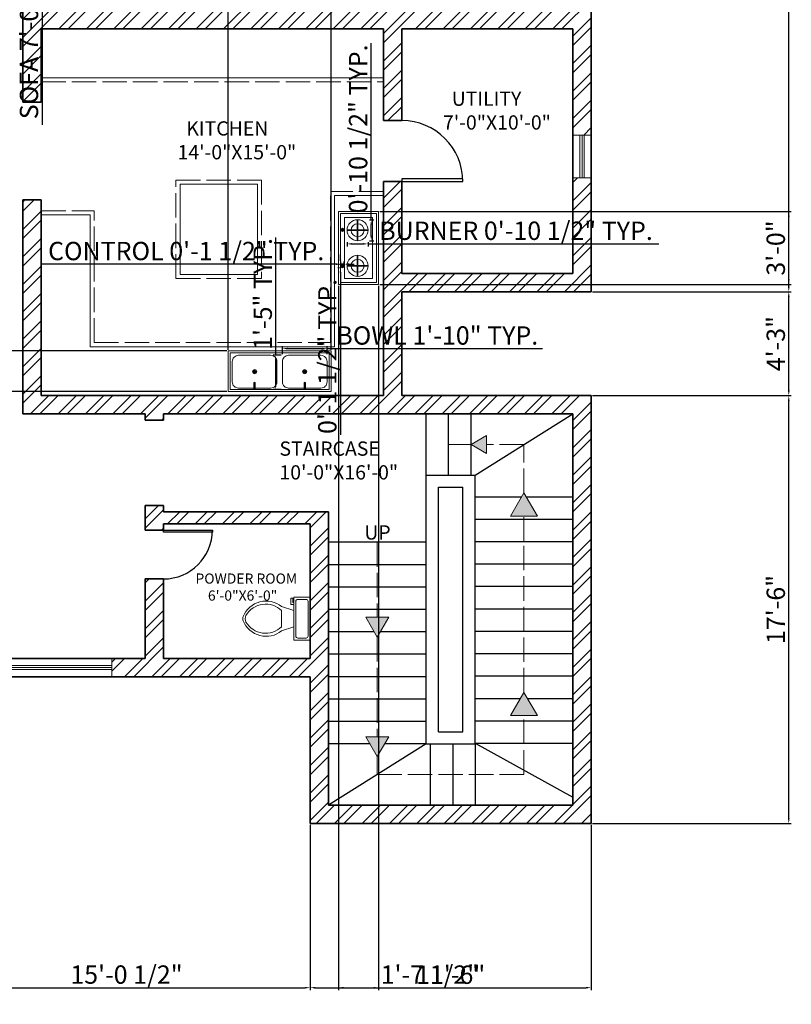
# Model space of a CAD drawing. Units: inches. Extents: x 416 to 1422, y 799 to 1634.
# Tile 4 of 5: x 1043 to 1422, y 799 to 1283. Entities that reach past the tile are written whole.
import ezdxf

# ---------------------------------------------------------------- set-up
doc = ezdxf.new("R2010")
doc.units = ezdxf.units.IN
doc.linetypes.add('ACAD_ISO02W100', pattern=[15, 12, -3])
for name, color, linetype, lineweight in [('A-ANNO-DIMS', 2, 'Continuous', 18), ('A-ANNO-STRS-PATH', 7, 'ACAD_ISO02W100', 18), ('A-ANNO-SYMB', 7, 'Continuous', 18), ('A-ANNO-TEXT', 7, 'Continuous', 18), ('A-AREA-IDEN', 7, 'Continuous', 18), ('A-DOOR', 4, 'Continuous', 25), ('A-EQPM', 9, 'Continuous', 18), ('A-FLOR-CASE', 8, 'Continuous', 18), ('A-FLOR-CASE-HIDN', 8, 'ACAD_ISO02W100', 13), ('A-FLOR-FIXT', 9, 'Continuous', 18), ('A-FLOR-STRS', 7, 'Continuous', 25), ('A-GLAZ', 244, 'Continuous', 18), ('A-WALL', 7, 'Continuous', 35), ('A-WALL-PATT', 252, 'Continuous', 13)]:
    doc.layers.add(name, color=color, linetype=linetype, lineweight=lineweight)
doc.styles.get("Standard").update_dxf_attribs({"font": 'arial.ttf'})
doc.dimstyles.new('ISO-25', dxfattribs={"dimtxt": 9, "dimasz": 2.5, "dimexe": 1.25, "dimexo": 0.625, "dimtad": 1, "dimlunit": 3, "dimtxsty": 'Standard', "dimcen": 2.5, "dimadec": 0, "dimazin": 0, "dimtfac": 1, "dimtmove": 0, "dimatfit": 3, "dimfxl": 1, "dimarcsym": 0})

# ---------------------------------------------------------------- blocks, each defined once
blk = doc.blocks.new('*U3')
for p, q in [((-40, 0), (-40, 6)), ((0, 0), (0, 6))]:
    blk.add_line(p, q)
blk.add_lwpolyline([(0, 0), (0, -40), (-1.75, -40), (-1.75, 0)], close=True)
blk.add_arc((0, 0), 40, 180, 270)
blk = doc.blocks.new('*U7')
for p, q in [((9.5, -6), (9.5, -2)), ((-10, -8.5), (-8, -8.5)), ((-10, -9.5), (-10, -8.5)), ((-7, -9.5), (-10, -9.5)), ((-8, -8.5), (-8, -8)), ((-7, -8), (-7, -9.5)), ((-4, -8), (-6, -14)), ((4, -8), (6, -14)), ((4, -14), (-4, -14))]:
    blk.add_line(p, q)
blk.add_lwpolyline([(10.5, -8), (10.5, 0), (-10.5, 0), (-10.5, -8)], close=True)
for points in [[(-9.5, -2), (-9.5, -6)], [(8.5, -1), (-8.5, -1)], [(-8.5, -7), (8.5, -7)]]:
    blk.add_lwpolyline(points)
for centre, radius, start, end in [((-8.62, -1.88), 0.884, 81.8699, 188.1301), ((8.62, -1.88), 0.884, 351.8699, 98.1301), ((-8.62, -6.12), 0.884, 171.8699, 278.1301), ((8.62, -6.12), 0.884, 261.8699, 8.1301), ((3.52, -21.58), 12.17, 141.4691, 247.9714), ((4.2, -21.82), 11.33, 136.3677, 238.9468), ((-3.52, -21.58), 12.17, 292.0284, 38.5307), ((-4.2, -21.82), 11.33, 301.053, 43.6321), ((0, -27.88), 4, 245.7318, 294.2682), ((0, -29), 4, 254.8605, 285.1395)]:
    blk.add_arc(centre, radius, start, end)
blk = doc.blocks.new('*U9')
for p, q in [((0, 0), (0, 6)), ((40, 0), (40, 6))]:
    blk.add_line(p, q)
blk.add_lwpolyline([(0, 0), (0, -40), (1.75, -40), (1.75, 0)], close=True)
blk.add_arc((0, 0), 40, 270, 360)
blk = doc.blocks.new('WIN-21IN')
for p, q in [((21, 5.5), (0, 5.5)), ((21, 4.5), (0, 4.5)), ((21, 3.5), (0, 3.5))]:
    blk.add_line(p, q)
blk.add_lwpolyline([(21, 9), (21, 0), (0, 0), (0, 9)], close=True)
blk = doc.blocks.new('WIN-60IN')
for p, q in [((3.5, 60), (3.5, 0)), ((4.5, 60), (4.5, 0)), ((5.5, 60), (5.5, 0))]:
    blk.add_line(p, q)
blk.add_lwpolyline([(0, 60), (9, 60), (9, 0), (0, 0)], close=True)
blk = doc.blocks.new('SINK-BOWL-WITH-DRAIN')
for p, q in [((10.95, 9.8), (10.95, 7.77)), ((9.94, 8.78), (11.97, 8.78)), ((10.22, 9.49), (11.68, 8.08)), ((11.67, 9.5), (10.23, 8.07)), ((10.71, 0), (10.71, 2.96)), ((10.81, 0), (10.81, 2.87)), ((11.21, 0), (11.21, 2.86)), ((11.31, 0), (11.31, 2.94))]:
    blk.add_line(p, q)
blk.add_lwpolyline([(10.71, 0.74), (3, 0.74, -0.414214), (0, 3.74), (0, 13.82, -0.414214), (3, 16.82), (18.91, 16.82, -0.414214), (21.91, 13.82), (21.91, 3.74, -0.414214), (18.91, 0.74), (11.31, 0.74)], format="xyb")
for centre, radius in [((10.95, 8.78), 1.02), ((10.95, 8.78), 0.616), ((11.02, 3.19), 0.381), ((11.02, 3.19), 0.181)]:
    blk.add_circle(centre, radius)
blk = doc.blocks.new('COOKTOP-BURNER')
for p, q in [((4.97, 10.34), (4.97, 5.37)), ((5.37, 10.34), (5.37, 5.37)), ((4.97, 5.37), (0, 5.37)), ((4.97, 4.97), (0, 4.97)), ((3.97, 5.37), (3.97, 4.97)), ((5.37, 6.37), (4.97, 6.37)), ((4.97, 4.97), (4.97, 0)), ((10.34, 5.37), (5.37, 5.37)), ((10.34, 4.97), (5.37, 4.97)), ((5.37, 4.97), (5.37, 0)), ((6.37, 5.37), (6.37, 4.97)), ((5.37, 3.97), (4.97, 3.97))]:
    blk.add_line(p, q)
for radius in [5.17, 3.17]:
    blk.add_circle((5.17, 5.17), radius)
blk = doc.blocks.new('COOKTOP-CONTROL')
for p, q in [((0.56, 1.39), (0.56, 0.13)), ((0.96, 1.39), (0.96, 0.13))]:
    blk.add_line(p, q)
for radius in [0.761, 0.661]:
    blk.add_circle((0.76, 0.76), radius)
blk = doc.blocks.new('*D27')
at = {"layer": 'A-ANNO-DIMS', "color": 0, "lineweight": -2, "transparency": 16777216}
for p, q in [((1042.27, 1411.23), (1055.49, 1411.23)), ((1054.24, 1408.73), (1054.24, 1329.73)), ((1042.27, 1327.23), (1055.49, 1327.23)), ((1054.24, 1327.23), (1054.24, 1230.94))]:
    blk.add_line(p, q, dxfattribs=at)
at = {"layer": 'A-ANNO-DIMS', "color": 0, "transparency": 16777216}
for points in [[(1053.83, 1408.73), (1054.66, 1408.73), (1054.24, 1411.23)], [(1053.83, 1329.73), (1054.66, 1329.73), (1054.24, 1327.23)]]:
    blk.add_solid(points, dxfattribs=at)
at = {"layer": 'Defpoints', "color": 0, "transparency": 16777216}
for p in [(1041.64, 1411.23), (1041.64, 1327.23), (1054.24, 1327.23)]:
    blk.add_point(p, dxfattribs=at)
at = {"layer": 'A-ANNO-DIMS', "color": 0, "transparency": 16777216, "insert": (1048.96, 1277.83), "char_height": 9, "attachment_point": 5, "rotation": 90}
blk.add_mtext('SOFA 7\'-0" TYP.', dxfattribs=at)
blk = doc.blocks.new('*D35')
at = {"layer": 'A-ANNO-DIMS', "color": 0, "lineweight": -2, "transparency": 16777216}
for p, q in [((1172.23, 1118.41), (1172.23, 1122.32)), ((1194.14, 1118.41), (1194.14, 1122.32)), ((1174.73, 1121.07), (1191.64, 1121.07)), ((1194.14, 1121.07), (1299.86, 1121.07))]:
    blk.add_line(p, q, dxfattribs=at)
at = {"layer": 'A-ANNO-DIMS', "color": 0, "transparency": 16777216}
for points in [[(1174.73, 1121.48), (1174.73, 1120.65), (1172.23, 1121.07)], [(1191.64, 1121.48), (1191.64, 1120.65), (1194.14, 1121.07)]]:
    blk.add_solid(points, dxfattribs=at)
at = {"layer": 'Defpoints', "color": 0, "transparency": 16777216}
for p in [(1172.23, 1117.78), (1194.14, 1121.07), (1194.14, 1117.78)]:
    blk.add_point(p, dxfattribs=at)
at = {"layer": 'A-ANNO-DIMS', "color": 0, "transparency": 16777216, "insert": (1248.25, 1126.35), "char_height": 9, "attachment_point": 5}
blk.add_mtext('BOWL 1\'-10" TYP.', dxfattribs=at)
blk = doc.blocks.new('*D36')
at = {"layer": 'A-ANNO-DIMS', "color": 0, "lineweight": -2, "transparency": 16777216}
for p, q in [((1168.94, 1117.78), (1168.94, 1175.54)), ((1171.6, 1117.78), (1167.69, 1117.78)), ((1168.94, 1103.46), (1168.94, 1115.28)), ((1171.6, 1100.96), (1167.69, 1100.96))]:
    blk.add_line(p, q, dxfattribs=at)
at = {"layer": 'A-ANNO-DIMS', "color": 0, "transparency": 16777216}
for points in [[(1168.53, 1115.28), (1169.36, 1115.28), (1168.94, 1117.78)], [(1168.53, 1103.46), (1169.36, 1103.46), (1168.94, 1100.96)]]:
    blk.add_solid(points, dxfattribs=at)
at = {"layer": 'Defpoints', "color": 0, "transparency": 16777216}
for p in [(1168.94, 1117.78), (1172.23, 1117.78), (1172.23, 1100.96)]:
    blk.add_point(p, dxfattribs=at)
at = {"layer": 'A-ANNO-DIMS', "color": 0, "transparency": 16777216, "insert": (1163.72, 1147.91), "char_height": 9, "attachment_point": 5, "rotation": 90}
blk.add_mtext('1\'-5" TYP.', dxfattribs=at)
blk = doc.blocks.new('*D37')
at = {"layer": 'A-ANNO-DIMS', "color": 0, "lineweight": -2, "transparency": 16777216}
for p, q in [((1203.95, 1173.39), (1203.95, 1171.22)), ((1206.45, 1172.47), (1211.78, 1172.47)), ((1214.28, 1173.39), (1214.28, 1171.22)), ((1214.28, 1172.47), (1357.04, 1172.47))]:
    blk.add_line(p, q, dxfattribs=at)
at = {"layer": 'A-ANNO-DIMS', "color": 0, "transparency": 16777216}
for points in [[(1206.45, 1172.88), (1206.45, 1172.05), (1203.95, 1172.47)], [(1211.78, 1172.88), (1211.78, 1172.05), (1214.28, 1172.47)]]:
    blk.add_solid(points, dxfattribs=at)
at = {"layer": 'Defpoints', "color": 0, "transparency": 16777216}
for p in [(1203.95, 1174.02), (1214.28, 1174.02), (1214.28, 1172.47)]:
    blk.add_point(p, dxfattribs=at)
at = {"layer": 'A-ANNO-DIMS', "color": 0, "transparency": 16777216, "insert": (1286.91, 1177.75), "char_height": 9, "attachment_point": 5}
blk.add_mtext('BURNER 0\'-10 1/2" TYP.', dxfattribs=at)
blk = doc.blocks.new('*D38')
at = {"layer": 'A-ANNO-DIMS', "color": 0, "lineweight": -2, "transparency": 16777216}
for p, q in [((1215.83, 1184.35), (1215.83, 1270.93)), ((1214.91, 1184.35), (1217.08, 1184.35)), ((1215.83, 1176.52), (1215.83, 1181.85)), ((1214.91, 1174.02), (1217.08, 1174.02))]:
    blk.add_line(p, q, dxfattribs=at)
at = {"layer": 'A-ANNO-DIMS', "color": 0, "transparency": 16777216}
for points in [[(1215.42, 1181.85), (1216.25, 1181.85), (1215.83, 1184.35)], [(1215.42, 1176.52), (1216.25, 1176.52), (1215.83, 1174.02)]]:
    blk.add_solid(points, dxfattribs=at)
at = {"layer": 'Defpoints', "color": 0, "transparency": 16777216}
for p in [(1214.28, 1184.35), (1215.83, 1184.35), (1214.28, 1174.02)]:
    blk.add_point(p, dxfattribs=at)
at = {"layer": 'A-ANNO-DIMS', "color": 0, "transparency": 16777216, "insert": (1210.56, 1228.89), "char_height": 9, "attachment_point": 5, "rotation": 90}
blk.add_mtext('0\'-10 1/2" TYP.', dxfattribs=at)
blk = doc.blocks.new('*D39')
at = {"layer": 'A-ANNO-DIMS', "color": 0, "lineweight": -2, "transparency": 16777216}
for p, q in [((1198.45, 1162.52), (1054, 1162.52)), ((1200.95, 1162.91), (1200.95, 1163.77)), ((1202.47, 1162.52), (1200.95, 1162.52)), ((1202.47, 1162.91), (1202.47, 1163.77)), ((1204.97, 1162.52), (1207.47, 1162.52))]:
    blk.add_line(p, q, dxfattribs=at)
at = {"layer": 'A-ANNO-DIMS', "color": 0, "transparency": 16777216}
for points in [[(1198.45, 1162.93), (1198.45, 1162.1), (1200.95, 1162.52)], [(1204.97, 1162.93), (1204.97, 1162.1), (1202.47, 1162.52)]]:
    blk.add_solid(points, dxfattribs=at)
at = {"layer": 'Defpoints', "color": 0, "transparency": 16777216}
for p in [(1200.95, 1162.52), (1200.95, 1162.29), (1202.47, 1162.29)]:
    blk.add_point(p, dxfattribs=at)
at = {"layer": 'A-ANNO-DIMS', "color": 0, "transparency": 16777216, "insert": (1124.98, 1167.8), "char_height": 9, "attachment_point": 5}
blk.add_mtext('CONTROL 0\'-1 1/2" TYP.', dxfattribs=at)
blk = doc.blocks.new('*D40')
at = {"layer": 'A-ANNO-DIMS', "color": 0, "lineweight": -2, "transparency": 16777216}
for p, q in [((1200.72, 1164.79), (1200.72, 1167.29)), ((1200.32, 1162.29), (1199.47, 1162.29)), ((1200.32, 1160.77), (1199.47, 1160.77)), ((1200.72, 1162.29), (1200.72, 1160.77)), ((1200.72, 1158.27), (1200.72, 1078.69))]:
    blk.add_line(p, q, dxfattribs=at)
at = {"layer": 'A-ANNO-DIMS', "color": 0, "transparency": 16777216}
for points in [[(1200.3, 1164.79), (1201.13, 1164.79), (1200.72, 1162.29)], [(1200.3, 1158.27), (1201.13, 1158.27), (1200.72, 1160.77)]]:
    blk.add_solid(points, dxfattribs=at)
at = {"layer": 'Defpoints', "color": 0, "transparency": 16777216}
for p in [(1200.72, 1160.77), (1200.95, 1162.29), (1200.95, 1160.77)]:
    blk.add_point(p, dxfattribs=at)
at = {"layer": 'A-ANNO-DIMS', "color": 0, "transparency": 16777216, "insert": (1195.44, 1117.23), "char_height": 9, "attachment_point": 5, "rotation": 90}
blk.add_mtext('0\'-1 1/2" TYP.', dxfattribs=at)
blk = doc.blocks.new('*D46')
at = {"layer": 'A-ANNO-DIMS', "color": 0, "lineweight": -2, "transparency": 16777216}
for p, q in [((1185.82, 887.39), (1185.82, 806.13)), ((1005.49, 855.39), (1005.49, 806.13)), ((1007.99, 807.38), (1183.32, 807.38))]:
    blk.add_line(p, q, dxfattribs=at)
at = {"layer": 'A-ANNO-DIMS', "color": 0, "transparency": 16777216}
for points in [[(1007.99, 807.79), (1007.99, 806.96), (1005.49, 807.38)], [(1183.32, 807.79), (1183.32, 806.96), (1185.82, 807.38)]]:
    blk.add_solid(points, dxfattribs=at)
at = {"layer": 'Defpoints', "color": 0, "transparency": 16777216}
for p in [(1185.82, 888.01), (1005.49, 856.01), (1185.82, 807.38)]:
    blk.add_point(p, dxfattribs=at)
at = {"layer": 'A-ANNO-DIMS', "color": 0, "transparency": 16777216, "insert": (1095.65, 812.65), "char_height": 9, "attachment_point": 5}
blk.add_mtext('15\'-0 1/2"', dxfattribs=at)
blk = doc.blocks.new('*D47')
at = {"layer": 'A-ANNO-DIMS', "color": 0, "lineweight": -2, "transparency": 16777216}
for p, q in [((1185.82, 887.39), (1185.82, 806.13)), ((1323.82, 887.39), (1323.82, 806.13)), ((1188.32, 807.38), (1321.32, 807.38))]:
    blk.add_line(p, q, dxfattribs=at)
at = {"layer": 'A-ANNO-DIMS', "color": 0, "transparency": 16777216}
for points in [[(1188.32, 807.79), (1188.32, 806.96), (1185.82, 807.38)], [(1321.32, 807.79), (1321.32, 806.96), (1323.82, 807.38)]]:
    blk.add_solid(points, dxfattribs=at)
at = {"layer": 'Defpoints', "color": 0, "transparency": 16777216}
for p in [(1185.82, 888.01), (1323.82, 888.01), (1323.82, 807.38)]:
    blk.add_point(p, dxfattribs=at)
at = {"layer": 'A-ANNO-DIMS', "color": 0, "transparency": 16777216, "insert": (1254.82, 812.6), "char_height": 9, "attachment_point": 5}
blk.add_mtext('11\'-6"', dxfattribs=at)
blk = doc.blocks.new('*D48')
at = {"layer": 'A-ANNO-DIMS', "color": 0, "lineweight": -2, "transparency": 16777216}
for p, q in [((1324.44, 1098.01), (1422.07, 1098.01)), ((1420.82, 890.51), (1420.82, 1095.51)), ((1324.44, 888.01), (1422.07, 888.01))]:
    blk.add_line(p, q, dxfattribs=at)
at = {"layer": 'A-ANNO-DIMS', "color": 0, "transparency": 16777216}
for points in [[(1420.4, 1095.51), (1421.24, 1095.51), (1420.82, 1098.01)], [(1420.4, 890.51), (1421.24, 890.51), (1420.82, 888.01)]]:
    blk.add_solid(points, dxfattribs=at)
at = {"layer": 'Defpoints', "color": 0, "transparency": 16777216}
for p in [(1323.82, 1098.01), (1420.82, 1098.01), (1323.82, 888.01)]:
    blk.add_point(p, dxfattribs=at)
at = {"layer": 'A-ANNO-DIMS', "color": 0, "transparency": 16777216, "insert": (1415.6, 993.01), "char_height": 9, "attachment_point": 5, "rotation": 90}
blk.add_mtext('17\'-6"', dxfattribs=at)
blk = doc.blocks.new('*D49')
at = {"layer": 'A-ANNO-DIMS', "color": 0, "lineweight": -2, "transparency": 16777216}
for p, q in [((1324.44, 1149.01), (1422.07, 1149.01)), ((1420.82, 1100.51), (1420.82, 1146.51)), ((1324.44, 1098.01), (1422.07, 1098.01))]:
    blk.add_line(p, q, dxfattribs=at)
at = {"layer": 'A-ANNO-DIMS', "color": 0, "transparency": 16777216}
for points in [[(1420.4, 1146.51), (1421.24, 1146.51), (1420.82, 1149.01)], [(1420.4, 1100.51), (1421.24, 1100.51), (1420.82, 1098.01)]]:
    blk.add_solid(points, dxfattribs=at)
at = {"layer": 'Defpoints', "color": 0, "transparency": 16777216}
for p in [(1323.82, 1149.01), (1420.82, 1149.01), (1323.82, 1098.01)]:
    blk.add_point(p, dxfattribs=at)
at = {"layer": 'A-ANNO-DIMS', "color": 0, "transparency": 16777216, "insert": (1415.6, 1123.51), "char_height": 9, "attachment_point": 5, "rotation": 90}
blk.add_mtext('4\'-3"', dxfattribs=at)
blk = doc.blocks.new('*D50')
at = {"layer": 'A-ANNO-DIMS', "color": 0, "lineweight": -2, "transparency": 16777216}
for p, q in [((1324.44, 1569.01), (1422.07, 1569.01)), ((1420.82, 1151.51), (1420.82, 1566.51)), ((1324.44, 1149.01), (1422.07, 1149.01))]:
    blk.add_line(p, q, dxfattribs=at)
at = {"layer": 'A-ANNO-DIMS', "color": 0, "transparency": 16777216}
for points in [[(1420.4, 1566.51), (1421.24, 1566.51), (1420.82, 1569.01)], [(1420.4, 1151.51), (1421.24, 1151.51), (1420.82, 1149.01)]]:
    blk.add_solid(points, dxfattribs=at)
at = {"layer": 'Defpoints', "color": 0, "transparency": 16777216}
for p in [(1323.82, 1569.01), (1420.82, 1569.01), (1323.82, 1149.01)]:
    blk.add_point(p, dxfattribs=at)
at = {"layer": 'A-ANNO-DIMS', "color": 0, "transparency": 16777216, "insert": (1415.6, 1359.01), "char_height": 9, "attachment_point": 5, "rotation": 90}
blk.add_mtext('35\'-0"', dxfattribs=at)
blk = doc.blocks.new('*D54')
at = {"layer": 'A-ANNO-DIMS', "color": 0, "lineweight": -2, "transparency": 16777216}
for p, q in [((1199.73, 1151.87), (1199.73, 806.13)), ((1219.46, 1151.87), (1219.46, 806.13)), ((1202.23, 807.38), (1216.96, 807.38)), ((1219.46, 807.38), (1267.26, 807.38))]:
    blk.add_line(p, q, dxfattribs=at)
at = {"layer": 'A-ANNO-DIMS', "color": 0, "transparency": 16777216}
for points in [[(1202.23, 807.79), (1202.23, 806.96), (1199.73, 807.38)], [(1216.96, 807.79), (1216.96, 806.96), (1219.46, 807.38)]]:
    blk.add_solid(points, dxfattribs=at)
at = {"layer": 'Defpoints', "color": 0, "transparency": 16777216}
for p in [(1199.73, 1152.5), (1219.46, 1152.5), (1219.46, 807.38)]:
    blk.add_point(p, dxfattribs=at)
at = {"layer": 'A-ANNO-DIMS', "color": 0, "transparency": 16777216, "insert": (1244.61, 812.65), "char_height": 9, "attachment_point": 5}
blk.add_mtext('1\'-7 1/2"', dxfattribs=at)
blk = doc.blocks.new('*D55')
at = {"layer": 'A-ANNO-DIMS', "color": 0, "lineweight": -2, "transparency": 16777216}
for p, q in [((1220.08, 1188.39), (1422.07, 1188.39)), ((1420.82, 1155), (1420.82, 1185.89)), ((1220.08, 1152.5), (1422.07, 1152.5))]:
    blk.add_line(p, q, dxfattribs=at)
at = {"layer": 'A-ANNO-DIMS', "color": 0, "transparency": 16777216}
for points in [[(1420.4, 1185.89), (1421.24, 1185.89), (1420.82, 1188.39)], [(1420.4, 1155), (1421.24, 1155), (1420.82, 1152.5)]]:
    blk.add_solid(points, dxfattribs=at)
at = {"layer": 'Defpoints', "color": 0, "transparency": 16777216}
for p in [(1219.46, 1188.39), (1420.82, 1188.39), (1219.46, 1152.5)]:
    blk.add_point(p, dxfattribs=at)
at = {"layer": 'A-ANNO-DIMS', "color": 0, "transparency": 16777216, "insert": (1415.6, 1170.44), "char_height": 9, "attachment_point": 5, "rotation": 90}
blk.add_mtext('3\'-0"', dxfattribs=at)
blk = doc.blocks.new('*D56')
at = {"layer": 'A-ANNO-DIMS', "color": 0, "lineweight": -2, "transparency": 16777216}
for p, q in [((1145.53, 1120.54), (1145.53, 1616.26)), ((1148.03, 1615.01), (1193.73, 1615.01)), ((1196.23, 1120.54), (1196.23, 1616.26))]:
    blk.add_line(p, q, dxfattribs=at)
at = {"layer": 'A-ANNO-DIMS', "color": 0, "transparency": 16777216}
for points in [[(1148.03, 1615.43), (1148.03, 1614.6), (1145.53, 1615.01)], [(1193.73, 1615.43), (1193.73, 1614.6), (1196.23, 1615.01)]]:
    blk.add_solid(points, dxfattribs=at)
at = {"layer": 'Defpoints', "color": 0, "transparency": 16777216}
for p in [(1196.23, 1615.01), (1145.53, 1119.92), (1196.23, 1119.92)]:
    blk.add_point(p, dxfattribs=at)
at = {"layer": 'A-ANNO-DIMS', "color": 0, "transparency": 16777216, "insert": (1170.88, 1620.29), "char_height": 9, "attachment_point": 5}
blk.add_mtext('4\'-2 1/2"', dxfattribs=at)
blk = doc.blocks.new('*D57')
at = {"layer": 'A-ANNO-DIMS', "color": 0, "lineweight": -2, "transparency": 16777216}
for p, q in [((434.25, 1119.92), (434.25, 1146.74)), ((1144.9, 1119.92), (433, 1119.92)), ((434.25, 1102.46), (434.25, 1117.42)), ((1144.9, 1099.96), (433, 1099.96))]:
    blk.add_line(p, q, dxfattribs=at)
at = {"layer": 'A-ANNO-DIMS', "color": 0, "transparency": 16777216}
for points in [[(433.83, 1117.42), (434.67, 1117.42), (434.25, 1119.92)], [(433.83, 1102.46), (434.67, 1102.46), (434.25, 1099.96)]]:
    blk.add_solid(points, dxfattribs=at)
at = {"layer": 'Defpoints', "color": 0, "transparency": 16777216}
for p in [(434.25, 1119.92), (1145.53, 1119.92), (1145.53, 1099.96)]:
    blk.add_point(p, dxfattribs=at)
at = {"layer": 'A-ANNO-DIMS', "color": 0, "transparency": 16777216, "insert": (429.03, 1134.58), "char_height": 9, "attachment_point": 5, "rotation": 90}
blk.add_mtext('1\'-8"', dxfattribs=at)

msp = doc.modelspace()

# ---------------------------------------------------------------- hatches: boundary and pattern name
at = {"layer": 'A-ANNO-SYMB'}
h = msp.add_hatch(color=256, dxfattribs=at)
h.dxf.hatch_style = 1
h.paths.add_polyline_path([(1224.457, 989.211), (1213.183, 989.211), (1218.82, 979.448)])
h.paths.add_polyline_path([(1224.457, 930.584), (1213.183, 930.584), (1218.82, 920.821)])
h.paths.add_polyline_path([(1290.82, 952.305), (1284.259, 940.942), (1297.38, 940.942)])
h.paths.add_polyline_path([(1290.82, 1050.204), (1284.259, 1038.841), (1297.38, 1038.841)])
h.paths.add_polyline_path([(1272.477, 1078.434), (1264.82, 1074.013), (1272.477, 1069.591)])
at = {"layer": 'A-WALL-PATT'}
h = msp.add_hatch(dxfattribs=at)
h.set_pattern_fill('ANSI32', color=256)
h.paths.add_polyline_path([(695.32, 1569.013), (607.303, 1569.013), (607.303, 1560.013), (660.82, 1560.013), (660.82, 1419.013), (657.82, 1419.013), (657.82, 1413.013), (669.82, 1413.013), (669.82, 1446.013), (672.82, 1446.013), (672.82, 1452.013), (669.82, 1452.013), (669.82, 1560.013), (695.32, 1560.013)])
h.paths.add_polyline_path([(1323.82, 1311.283), (1314.82, 1311.283), (1314.82, 1287.013), (1242.82, 1287.013), (1242.82, 1383.013), (1245.82, 1383.013), (1245.82, 1392.013), (1236.82, 1392.013), (1236.82, 1339.513), (1158.82, 1339.513), (1158.82, 1431.013), (1149.82, 1431.013), (1149.82, 1287.013), (1044.82, 1287.013), (1044.82, 1242.013), (1053.82, 1242.013), (1053.82, 1278.013), (1221.82, 1278.013), (1221.82, 1233.013), (1230.82, 1233.013), (1230.82, 1278.013), (1314.82, 1278.013), (1314.82, 1225.894), (1323.82, 1225.894)])
h.paths.add_polyline_path([(1158.82, 1287.013), (1158.82, 1333.513), (1236.82, 1333.513), (1236.82, 1287.013)], flags=16)
h.paths.add_polyline_path([(1323.82, 1569.013), (1283.747, 1569.013), (1283.747, 1560.013), (1314.82, 1560.013), (1314.82, 1392.013), (1275.82, 1392.013), (1275.82, 1383.013), (1314.82, 1383.013), (1314.82, 1332.283), (1323.82, 1332.283)])
h.paths.add_polyline_path([(750.82, 1569.013), (716.32, 1569.013), (716.32, 1560.013), (741.82, 1560.013), (741.82, 1452.013), (702.82, 1452.013), (702.82, 1447.513), (702.82, 1446.013), (741.82, 1446.013), (741.82, 1287.013), (750.82, 1287.013)])
h.paths.add_polyline_path([(1158.82, 1560.013), (1223.747, 1560.013), (1223.747, 1569.013), (1149.82, 1569.013), (1149.82, 1467.013), (1158.82, 1467.013)])
h.paths.add_polyline_path([(1323.82, 1098.013), (1230.82, 1098.013), (1230.82, 1149.013), (1323.82, 1149.013), (1323.82, 1204.894), (1314.82, 1204.894), (1314.82, 1158.013), (1230.82, 1158.013), (1230.82, 1203.013), (1221.82, 1203.013), (1221.82, 1098.013), (1053.82, 1098.013), (1053.82, 1194.013), (1044.82, 1194.013), (1044.82, 1089.013), (1104.82, 1089.013), (1104.82, 1086.013), (1113.82, 1086.013), (1113.82, 1089.013), (1194.82, 1089.013), (1314.82, 1089.013), (1314.82, 897.013), (1194.82, 897.013), (1194.82, 1041.013), (1113.82, 1041.013), (1113.82, 1044.013), (1104.82, 1044.013), (1104.82, 1032.013), (1113.82, 1032.013), (1113.82, 1035.013), (1185.82, 1035.013), (1185.82, 969.013), (1113.82, 969.013), (1113.82, 1008.013), (1104.82, 1008.013), (1104.82, 969.013), (1088.452, 969.013), (1088.452, 960.013), (1185.82, 960.013), (1185.82, 888.013), (1323.82, 888.013)])

# ---------------------------------------------------------------- linework, layer by layer
at = {"layer": 'A-ANNO-STRS-PATH'}
for p, q in [((1264.82, 1074.013), (1253.82, 1074.013)), ((1290.82, 1074.013), (1272.477, 1074.013)), ((1290.82, 1050.204), (1290.82, 1074.013)), ((1290.82, 1026.395), (1290.82, 1038.841)), ((1218.82, 1026.013), (1218.82, 989.211)), ((1290.82, 952.305), (1290.82, 1026.395)), ((1218.82, 979.448), (1218.82, 930.584)), ((1290.82, 912.013), (1290.82, 940.942)), ((1218.82, 920.821), (1218.82, 912.013)), ((1218.82, 912.013), (1290.82, 912.013))]:
    msp.add_line(p, q, dxfattribs=at)
at = {"layer": 'A-ANNO-SYMB'}
for points in [[(1264.82, 1074.013), (1272.477, 1069.591), (1272.477, 1078.434)], [(1290.82, 1050.204), (1284.259, 1038.841), (1297.38, 1038.841)], [(1218.82, 979.448), (1224.457, 989.211), (1213.183, 989.211)], [(1290.82, 952.305), (1284.259, 940.942), (1297.38, 940.942)], [(1218.82, 920.821), (1224.457, 930.584), (1213.183, 930.584)]]:
    msp.add_lwpolyline(points, close=True, dxfattribs=at)
at = {"layer": 'A-EQPM'}
for points in [[(1199.726, 1188.394), (1219.46, 1188.394), (1219.46, 1152.496), (1199.726, 1152.496)], [(1200.726, 1187.394), (1218.46, 1187.394), (1218.46, 1153.496), (1200.726, 1153.496)], [(1202.726, 1185.394), (1216.46, 1185.394), (1216.46, 1155.496), (1202.726, 1155.496)]]:
    msp.add_lwpolyline(points, close=True, dxfattribs=at)
at = {"layer": 'A-FLOR-CASE'}
for p, q in [((1053.82, 1254.013), (1221.82, 1254.013)), ((1197.82, 1122.013), (1197.82, 1196.185)), ((1221.82, 1196.185), (1197.82, 1196.185)), ((1053.82, 1186.76), (1077.82, 1186.76)), ((1077.82, 1122.013), (1077.82, 1186.76)), ((1077.82, 1122.013), (1197.82, 1122.013))]:
    msp.add_line(p, q, dxfattribs=at)
msp.add_lwpolyline([(1121.959, 1201.774), (1159.95, 1201.774), (1159.95, 1157.434), (1121.959, 1157.434)], close=True, dxfattribs=at)
at = {"layer": 'A-FLOR-CASE-HIDN'}
for p, q in [((1053.82, 1252.013), (1221.82, 1252.013)), ((1221.82, 1198.185), (1195.82, 1198.185)), ((1195.82, 1124.013), (1195.82, 1198.185)), ((1053.82, 1188.76), (1079.82, 1188.76)), ((1079.82, 1124.013), (1079.82, 1188.76)), ((1079.82, 1124.013), (1195.82, 1124.013))]:
    msp.add_line(p, q, dxfattribs=at)
msp.add_lwpolyline([(1119.959, 1203.774), (1161.95, 1203.774), (1161.95, 1155.434), (1119.959, 1155.434)], close=True, dxfattribs=at)
at = {"layer": 'A-FLOR-FIXT'}
for points in [[(1145.527, 1119.918), (1196.227, 1119.918), (1196.227, 1099.958), (1145.527, 1099.958)], [(1146.527, 1118.918), (1195.227, 1118.918), (1195.227, 1100.958), (1146.527, 1100.958)]]:
    msp.add_lwpolyline(points, close=True, dxfattribs=at)
at = {"layer": 'A-FLOR-STRS'}
for p, q in [((1242.82, 1059.013), (1242.82, 1089.013)), ((1253.82, 1059.013), (1253.82, 1089.013)), ((1264.82, 1059.013), (1264.82, 1089.013)), ((1266.82, 1059.013), (1314.82, 1089.013)), ((1242.82, 927.013), (1242.82, 1059.013)), ((1242.82, 1059.013), (1266.82, 1059.013)), ((1266.82, 927.013), (1266.82, 1059.013)), ((1248.82, 933.013), (1248.82, 1053.013)), ((1248.82, 1053.013), (1260.82, 1053.013)), ((1260.82, 933.013), (1260.82, 1053.013)), ((1266.82, 1048.395), (1289.776, 1048.395)), ((1291.864, 1048.395), (1314.82, 1048.395)), ((1266.82, 1037.395), (1314.82, 1037.395)), ((1242.82, 1026.013), (1194.82, 1026.013)), ((1266.82, 1026.395), (1314.82, 1026.395)), ((1242.82, 1015.013), (1194.82, 1015.013)), ((1266.82, 1015.395), (1314.82, 1015.395)), ((1242.82, 1004.013), (1194.82, 1004.013)), ((1266.82, 1004.395), (1314.82, 1004.395)), ((1242.82, 993.013), (1194.82, 993.013)), ((1266.82, 993.395), (1314.82, 993.395)), ((1217.339, 982.013), (1194.82, 982.013)), ((1242.82, 982.013), (1220.3, 982.013)), ((1266.82, 982.395), (1314.82, 982.395)), ((1266.82, 971.395), (1314.82, 971.395)), ((1242.82, 971.013), (1194.82, 971.013)), ((1242.82, 960.013), (1194.82, 960.013)), ((1266.82, 960.395), (1314.82, 960.395)), ((1242.82, 949.013), (1194.82, 949.013)), ((1266.82, 949.395), (1289.14, 949.395)), ((1292.5, 949.395), (1314.82, 949.395)), ((1242.82, 938.013), (1194.82, 938.013)), ((1266.82, 938.395), (1314.82, 938.395)), ((1248.82, 933.013), (1260.82, 933.013)), ((1242.82, 927.013), (1194.82, 897.013)), ((1215.245, 927.013), (1194.82, 927.013)), ((1242.82, 927.013), (1222.395, 927.013)), ((1242.82, 927.013), (1266.82, 927.013)), ((1244.82, 927.013), (1244.82, 897.013)), ((1255.82, 927.013), (1255.82, 897.013)), ((1266.82, 927.395), (1314.82, 927.395)), ((1266.82, 927.395), (1314.82, 900.9)), ((1266.82, 927.013), (1266.82, 897.013))]:
    msp.add_line(p, q, dxfattribs=at)
at = {"layer": 'A-WALL'}
for p, q in [((1323.82, 1569.013), (1323.82, 1149.013)), ((1044.82, 1242.013), (1044.82, 1287.013)), ((1053.82, 1278.013), (1221.82, 1278.013)), ((1053.82, 1242.013), (1053.82, 1278.013)), ((1221.82, 1233.013), (1221.82, 1278.013)), ((1230.82, 1278.013), (1314.82, 1278.013)), ((1230.82, 1233.013), (1230.82, 1278.013)), ((1314.82, 1158.013), (1314.82, 1278.013)), ((1053.82, 1242.013), (1044.82, 1242.013)), ((1230.82, 1233.013), (1221.82, 1233.013)), ((1221.82, 1098.013), (1221.82, 1203.013)), ((1230.82, 1203.013), (1221.82, 1203.013)), ((1230.82, 1158.013), (1230.82, 1203.013)), ((1044.82, 1089.013), (1044.82, 1194.013)), ((1053.82, 1194.013), (1044.82, 1194.013)), ((1053.82, 1098.013), (1053.82, 1194.013)), ((1230.82, 1158.013), (1314.82, 1158.013)), ((1230.82, 1098.013), (1230.82, 1149.013)), ((1230.82, 1149.013), (1323.82, 1149.013)), ((1053.82, 1098.013), (1221.82, 1098.013)), ((1230.82, 1098.013), (1323.82, 1098.013)), ((1323.82, 1098.013), (1323.82, 888.013)), ((1044.82, 1089.013), (1104.82, 1089.013)), ((1104.82, 1086.013), (1104.82, 1089.013)), ((1113.82, 1089.013), (1194.82, 1089.013)), ((1113.82, 1086.013), (1113.82, 1089.013)), ((1194.82, 1089.013), (1314.82, 1089.013)), ((1314.82, 897.013), (1314.82, 1089.013)), ((1113.82, 1086.013), (1104.82, 1086.013)), ((1113.82, 1044.013), (1104.82, 1044.013)), ((1104.82, 1032.013), (1104.82, 1044.013)), ((1113.82, 1041.013), (1113.82, 1044.013)), ((1113.82, 1041.013), (1194.82, 1041.013)), ((1194.82, 897.013), (1194.82, 1041.013)), ((1113.82, 1035.013), (1185.82, 1035.013)), ((1113.82, 1032.013), (1113.82, 1035.013)), ((1185.82, 969.013), (1185.82, 1035.013)), ((1113.82, 1032.013), (1104.82, 1032.013)), ((1104.82, 969.013), (1104.82, 1008.013)), ((1113.82, 1008.013), (1104.82, 1008.013)), ((1113.82, 969.013), (1113.82, 1008.013)), ((977.602, 969.013), (1104.82, 969.013)), ((1113.82, 969.013), (1185.82, 969.013)), ((977.602, 960.013), (1185.82, 960.013)), ((1185.82, 888.013), (1185.82, 960.013)), ((1194.82, 897.013), (1314.82, 897.013)), ((1185.82, 888.013), (1323.82, 888.013))]:
    msp.add_line(p, q, dxfattribs=at)

# ---------------------------------------------------------------- block references
at = {"layer": 'A-DOOR', "rotation": 89.99999999999994}
for name, p, xscale, yscale, zscale in [('*U9', (1230.82, 1203.013), 0.7500000000000002, 0.7500000000000002, 0.7500000000000002), ('*U3', (1113.82, 1032.013), 0.5999999999999897, 0.5999999999999897, 0.5999999999999897)]:
    msp.add_blockref(name, p, dxfattribs=dict(at, xscale=xscale, yscale=yscale, zscale=zscale))
at = {"layer": 'A-EQPM'}
for name, p in [('COOKTOP-BURNER', (1203.948, 1174.018)), ('COOKTOP-CONTROL', (1200.946, 1178.601)), ('COOKTOP-BURNER', (1203.948, 1156.536))]:
    msp.add_blockref(name, p, dxfattribs=at)
at = {"layer": 'A-EQPM', "rotation": 180}
msp.add_blockref('COOKTOP-CONTROL', (1202.468, 1162.289), dxfattribs=at)
at = {"layer": 'A-FLOR-FIXT', "extrusion": (0, 0, -1), "zscale": -1}
msp.add_blockref('SINK-BOWL-WITH-DRAIN', (-1169.524, 1100.958), dxfattribs=at)
at = {"layer": 'A-FLOR-FIXT'}
msp.add_blockref('SINK-BOWL-WITH-DRAIN', (1172.23, 1100.958), dxfattribs=at)
at = {"layer": 'A-FLOR-FIXT', "rotation": 270}
msp.add_blockref('*U7', (1185.82, 988.503), dxfattribs=at)
at = {"layer": 'A-GLAZ'}
for name, p, rotation in [('WIN-21IN', (1323.819, 1204.894), 89.9999999999983), ('WIN-60IN', (1028.452, 969.012), 270.0000000000001)]:
    msp.add_blockref(name, p, dxfattribs=dict(at, rotation=rotation))

# ---------------------------------------------------------------- texts
at = {"layer": 'A-ANNO-TEXT', "insert": (1212.436, 1034.334), "char_height": 7, "attachment_point": 1}
msp.add_mtext_dynamic_manual_height_columns('UP ', width=14.18959, gutter_width=12.5, heights=[0], dxfattribs=at)
at = {"layer": 'A-AREA-IDEN', "attachment_point": 1}
for s, width, insert, char_height in [('  UTILITY        7\'-0"X10\'-0"', 49.74549, (1251.066, 1247.24), 7), ('   KITCHEN        14\'-0"X15\'-0"', 61.48634, (1118.614, 1232.648), 7), ('STAIRCASE          10\'-0"X16\'-0"', 56.28135, (1170.767, 1075.494), 7), ('POWDER ROOM       6\'-0"X6\'-0"', 54.28741, (1129.538, 1010.702), 5)]:
    msp.add_mtext_dynamic_manual_height_columns(s, width=width, gutter_width=12.5, heights=[0], dxfattribs=dict(at, insert=insert, char_height=char_height))

# ---------------------------------------------------------------- dimensions: what is measured, and where the dimension line sits
at = {"layer": 'A-ANNO-DIMS'}
for base, p1, p2, picture, middle in [((1196.227, 1615.013), (1145.527, 1119.918), (1196.227, 1119.918), '*D56', (1170.877, 1620.291)), ((1219.46, 807.375), (1199.726, 1152.496), (1219.46, 1152.496), '*D54', (1244.609, 812.654)), ((1185.82, 807.375), (1005.486, 856.013), (1185.82, 888.013), '*D46', (1095.653, 812.654)), ((1323.82, 807.375), (1185.82, 888.013), (1323.82, 888.013), '*D47', (1254.82, 812.596))]:
    dim = msp.add_linear_dim(base=base, p1=p1, p2=p2, dimstyle='ISO-25', override={"dimdec": 1, "dimlfac": 1, "dimrnd": 0, "dimzin": 1, "dimdsep": 46, "dimlunit": 4, "dimfrac": 2}, dxfattribs=at)
    dim.commit()
    dim.dimension.update_dxf_attribs({"geometry": picture, "text_midpoint": middle})
for base, p1, p2, picture, middle in [((1420.82, 1569.013), (1323.82, 1149.013), (1323.82, 1569.013), '*D50', (1415.597, 1359.013)), ((1420.82, 1188.394), (1219.46, 1152.496), (1219.46, 1188.394), '*D55', (1415.597, 1170.445)), ((434.249, 1119.918), (1145.527, 1099.958), (1145.527, 1119.918), '*D57', (429.029, 1134.581)), ((1420.82, 1149.013), (1323.82, 1098.013), (1323.82, 1149.013), '*D49', (1415.597, 1123.513)), ((1420.82, 1098.013), (1323.82, 888.013), (1323.82, 1098.013), '*D48', (1415.6, 993.013))]:
    dim = msp.add_linear_dim(base=base, p1=p1, p2=p2, angle=90, dimstyle='ISO-25', override={"dimdec": 1, "dimlfac": 1, "dimrnd": 0, "dimzin": 1, "dimdsep": 46, "dimlunit": 4, "dimfrac": 2}, dxfattribs=at)
    dim.commit()
    dim.dimension.update_dxf_attribs({"geometry": picture, "text_midpoint": middle})
for base, p1, p2, angle, text, picture, middle in [((1054.243, 1327.231), (1041.643, 1411.231), (1041.643, 1327.231), 270, 'SOFA <> TYP.', '*D27', (1048.961, 1277.835)), ((1215.835, 1184.354), (1214.284, 1174.018), (1214.284, 1184.354), 90, '<> TYP.', '*D38', (1210.556, 1228.891)), ((1200.946, 1162.517), (1202.468, 1162.289), (1200.946, 1162.289), 180, 'CONTROL <> TYP.', '*D39', (1124.975, 1167.799)), ((1168.944, 1117.781), (1172.23, 1100.958), (1172.23, 1117.781), 90, '<> TYP.', '*D36', (1163.724, 1147.912)), ((1200.717, 1160.766), (1200.946, 1162.289), (1200.946, 1160.766), 270, '<> TYP.', '*D40', (1195.439, 1117.226))]:
    dim = msp.add_linear_dim(base=base, p1=p1, p2=p2, angle=angle, text=text, dimstyle='ISO-25', override={"dimdec": 1, "dimlfac": 1, "dimrnd": 0, "dimzin": 1, "dimdsep": 46, "dimlunit": 4, "dimfrac": 2}, dxfattribs=at)
    dim.commit()
    dim.dimension.update_dxf_attribs({"geometry": picture, "text_midpoint": middle})
for base, p1, p2, text, picture, middle in [((1214.284, 1172.467), (1203.948, 1174.018), (1214.284, 1174.018), 'BURNER <> TYP.', '*D37', (1286.914, 1177.746)), ((1194.136, 1121.067), (1172.23, 1117.781), (1194.136, 1117.781), 'BOWL <> TYP.', '*D35', (1248.246, 1126.349))]:
    dim = msp.add_linear_dim(base=base, p1=p1, p2=p2, text=text, dimstyle='ISO-25', override={"dimdec": 1, "dimlfac": 1, "dimrnd": 0, "dimzin": 1, "dimdsep": 46, "dimlunit": 4, "dimfrac": 2}, dxfattribs=at)
    dim.commit()
    dim.dimension.update_dxf_attribs({"geometry": picture, "text_midpoint": middle})

doc.saveas('drawing.dxf')
